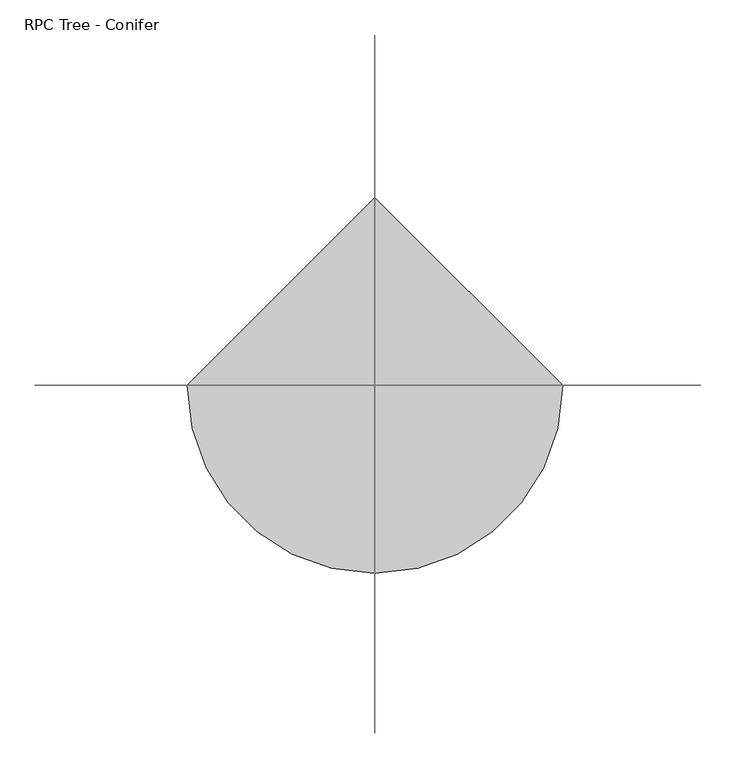
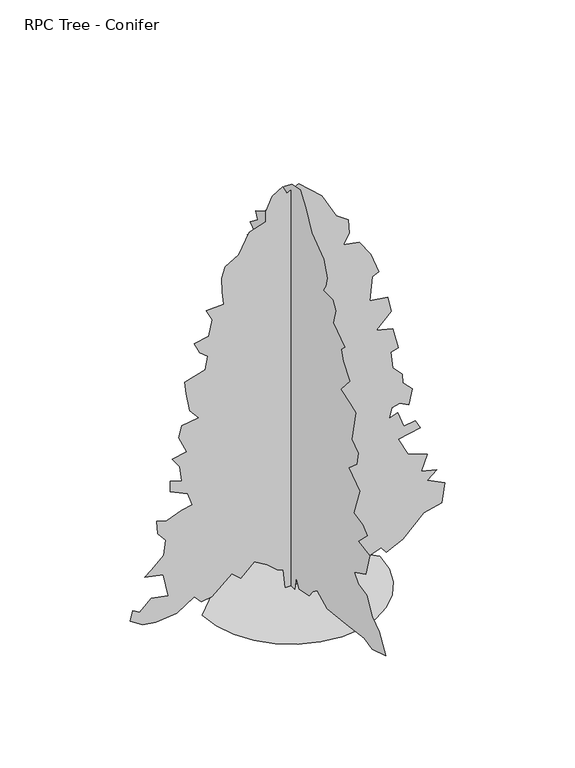
"""IFC4 building model written with IfcOpenShell, lengths in millimetres: geographic element geometry, RPC Tree - Conifer."""

from ifc_helpers import new_model, si_unit, origin, place, context, project, spatial, triangles, source, transform, mapped, element, save


def rpc_tree_conifer_9dfc94cb(model_context):
    return source(origin(), model_context, "Body", "Tessellation", [
        triangles([(0.1966724, 30.3730143, 2.21e-05), (0.196677, 46.8765628, 127.9026127), (0.1966796, 67.5060358, 185.6643395), (0.1966817, 141.7719332, 144.4061656), (0.1966847, 232.5410567, 107.2731397), (0.1966888, 335.6884489, 90.7695958), (0.1966936, 439.1223244, 95.1599346), (0.196692, 451.2137375, 24.7553998), (0.1966968, 525.4797712, 74.2660428), (0.1966987, 604.2812476, 22.1498153), (0.1967019, 661.6339605, 41.258946), (0.1967068, 773.0337742, 37.1330214), (0.1967106, 826.6693811, 86.6436667), (0.1967191, 942.1947424, 198.0422722), (0.196717, 872.0541109, 231.0490693), (0.1967148, 810.166028, 251.6794597), (0.1967121, 752.5176573, 246.8636199), (0.1967135, 740.0254692, 313.5675608), (0.196716, 756.5288223, 371.3302051), (0.1967205, 814.291503, 437.3437992), (0.1967183, 756.5288223, 449.7217501), (0.1967216, 801.9135521, 490.9809686), (0.196719, 731.7745193, 511.609833), (0.1967168, 657.5084856, 548.7436492), (0.1967174, 619.3261505, 625.1478155), (0.1967225, 715.2710936, 651.8910233), (0.1967254, 756.5288223, 689.0232771), (0.1967234, 702.8932154, 701.4011553), (0.1967209, 612.1237558, 755.038361), (0.1967249, 678.1373137, 788.0451399), (0.1967284, 683.4773947, 896.6957027), (0.1967253, 607.9967548, 907.6959034), (0.1967228, 541.9831607, 924.1993292), (0.1967255, 551.7215198, 999.3751911), (0.1967298, 632.118611, 1022.0385607), (0.1967329, 649.2560097, 1101.6127007), (0.1967296, 583.2424155, 1089.2348225), (0.1967301, 541.5533904, 1169.5343542), (0.1967339, 587.3678905, 1225.3890118), (0.1967327, 529.6052462, 1274.8992165), (0.1967366, 587.3678905, 1316.1584713), (0.1967383, 603.8712799, 1349.1651775), (0.1967356, 500.7239058, 1415.1803341), (0.1967363, 488.3459913, 1456.4379902), (0.1967412, 570.864501, 1497.697245), (0.1967412, 533.7307211, 1551.3406277), (0.1967386, 451.2137375, 1588.4652512), (0.1967428, 504.8493808, 1650.3547874), (0.1967418, 447.0867365, 1703.9843628), (0.1967401, 372.8222288, 1757.6291988), (0.1967419, 368.6952278, 1823.6488609), (0.1967455, 430.583347, 1852.5286388), (0.1967445, 385.2001433, 1885.5385426), (0.1967425, 331.562974, 1897.9133686), (0.1967471, 401.7035328, 1947.4129635), (0.1967455, 327.437499, 2005.18778), (0.1967476, 348.0663634, 2046.442384), (0.1967452, 261.422397, 2095.9572395), (0.1967443, 191.28182, 2170.2217472), (0.1967451, 145.0015871, 2265.4870079), (0.1967443, 59.2541866, 2368.2654728), (0.196743, -6.7601286, 2421.8950481), (0.1967397, -89.2778991, 2438.4), (0.196735, -147.040398, 2364.1354923), (0.1967289, -204.8027425, 2248.6162354), (0.196721, -324.4534879, 2161.9616409), (0.1967167, -357.4603031, 2067.0774616), (0.1967157, -340.9569137, 2009.3024998), (0.1967155, -320.3280493, 1972.1778763), (0.1967115, -411.0974725, 1972.1778763), (0.1967087, -439.9788128, 1922.663166), (0.1967072, -415.2229474, 1836.0238323), (0.1966997, -530.748236, 1757.6291988), (0.1967004, -493.6144561, 1724.6192951), (0.1966976, -514.2448465, 1662.7297588), (0.1966924, -580.2584407, 1584.3351254), (0.1966933, -489.4889812, 1481.1938919), (0.1966882, -585.0590198, 1451.3387375), (0.1966851, -638.021085, 1427.5582123), (0.1966813, -600.8873051, 1246.0178398), (0.1966772, -662.776914, 1200.63311), (0.1966756, -650.3990358, 1126.3670763), (0.196677, -572.0059648, 1056.2280436), (0.19667, -679.2803398, 981.9619371), (0.1966677, -617.3921843, 812.7995155), (0.1966632, -708.1616438, 796.2960897), (0.19666, -753.5463736, 759.1638359), (0.1966614, -662.776914, 668.3943764), (0.1966557, -778.3006765, 651.8910233), (0.1966535, -737.0429478, 515.7353079), (0.1966569, -625.6431341, 462.0996646), (0.1966537, -662.776914, 412.5894599), (0.1966494, -749.4193726, 396.0860704), (0.1966442, -803.0565783, 301.1896462), (0.1966395, -873.1971371, 251.6794597), (0.1966336, -935.08522, 144.4061656), (0.1966382, -803.0565783, 103.1472196), (0.1966424, -722.0818697, 121.6549744), (0.1966497, -545.8937505, 100.0198124), (0.1966574, -357.4603031, 78.3918175), (0.1966633, -258.438404, 127.9026127), (0.1966642, -217.1806752, 94.8953614), (0.1966645, -180.0468771, 49.5106453), (0.1966683, -81.0260499, 28.8813244), (0.1966712, -52.3611344, 81.269894), (0.1966695, -35.6413315, 2.01e-05), (-31.1375321, 8e-07, 2.21e-05), (-43.5151537, -1.27e-05, 111.3990688), (-76.522246, -1.22e-05, 123.7766926), (-134.2847449, -1.27e-05, 173.287951), (-208.5501882, -1.25e-05, 218.6726626), (-286.943223, 2e-06, 144.4061656), (-336.4534095, 1.4e-06, 189.7913405), (-451.9786981, 9.3e-06, 90.7695958), (-509.9897647, 1.13e-05, 83.5094103), (-550.9990711, 1.06e-05, 127.9026127), (-650.0210066, 1.65e-05, 61.888419), (-769.6717701, 2.94e-05, 49.5107997), (-843.9378038, 3.11e-05, 61.888419), (-914.0783627, 3.12e-05, 107.2731397), (-901.7004845, 2.82e-05, 165.0354751), (-860.4412296, 2.81e-05, 140.2802365), (-794.4260731, 1.45e-05, 202.1692732), (-699.5312113, 1.24e-05, 185.6643395), (-727.5164217, 7.2e-06, 321.9373624), (-831.559853, 9.3e-06, 342.4489011), (-794.4260731, 6.9e-06, 371.3302051), (-724.2870403, 1.9e-06, 437.3437992), (-711.9090895, -2.3e-06, 523.9877838), (-757.2938192, -3.4e-06, 577.6249532), (-765.5462952, -6.6e-06, 656.0164982), (-707.7836872, -7.6e-06, 639.5130724), (-621.1397026, -2.05e-05, 672.5198513), (-563.3769856, -2.28e-05, 684.8978022), (-588.132851, -2.54e-05, 759.1638359), (-687.2416271, -2.45e-05, 805.5818602), (-687.1532604, -2.74e-05, 870.5621235), (-621.1397026, -2.85e-05, 849.9332954), (-632.272526, -3.21e-05, 937.6303408), (-674.7768356, -3.35e-05, 998.4653629), (-592.258326, -3.67e-05, 1014.9687887), (-637.6430557, -3.98e-05, 1113.9891254), (-621.1397026, -4.32e-05, 1180.0042093), (-526.2447318, -5.56e-05, 1196.5076351), (-575.7549365, -5.67e-05, 1254.2702431), (-596.3838009, -6.11e-05, 1365.6685307), (-604.6362405, -6.4e-05, 1435.8091621), (-489.1109519, -6.91e-05, 1472.9414886), (-472.6075624, -7.29e-05, 1547.2105019), (-517.9922922, -7.32e-05, 1584.3351254), (-550.9990711, -7.52e-05, 1650.3547874), (-467.0983057, -8.72e-05, 1664.4822681), (-447.8516971, -9.19e-05, 1757.6291988), (-480.858476, -9.39e-05, 1823.6488609), (-381.8381029, -9.7e-05, 1827.763726), (-390.0890528, -0.0001003, 1906.1582142), (-394.2160538, -0.0001038, 1988.6828281), (-373.5856633, -0.0001072, 2050.5725098), (-297.1098262, -0.0001205, 2097.5878086), (-237.4315104, -0.0001273, 2211.4763512), (-142.5364396, -0.0001314, 2240.3561291), (-142.5364396, -0.0001342, 2302.2458107), (-105.4034228, -0.0001388, 2380.6404442), (-47.6410782, -0.0001422, 2417.7650677), (-22.8856807, -0.0001409, 2372.3803379), (43.128513, -0.0001532, 2405.3900963), (175.1564416, -0.0001518, 2285.7408588), (257.6749331, -0.0001388, 2137.2118435), (327.8155283, -0.0001475, 2087.6971333), (331.9410032, -0.0001351, 2005.18778), (298.934188, -0.0001315, 1947.4129635), (389.7036475, -0.0001335, 1930.9232723), (455.7172417, -0.0001312, 1836.0238323), (501.1019714, -0.0001272, 1716.3744495), (463.56887, -0.0001252, 1696.8520947), (447.4662918, -0.0001186, 1559.5853279), (550.6121398, -0.0001209, 1543.0805214), (571.2425303, -0.0001175, 1452.3125153), (484.5985456, -0.0001112, 1369.7956043), (579.4934801, -0.0001129, 1345.0397026), (612.5017124, -9.94e-05, 1217.1365358), (567.1155293, -9.76e-05, 1208.885586), (579.4934801, -9.36e-05, 1109.8636505), (634.0572281, -9.25e-05, 1050.2615473), (637.2560881, -9.03e-05, 998.4653629), (690.8932211, -8.95e-05, 944.8281572), (670.262867, -8.48e-05, 854.0587704), (620.7526623, -8.47e-05, 882.9400743), (575.3680052, -8.28e-05, 870.5621235), (558.8646157, -7.97e-05, 812.7995155), (608.3747841, -8.19e-05, 829.3028687), (641.381563, -7.86e-05, 734.4080069), (707.3966469, -8.12e-05, 746.785885), (736.2779509, -7.96e-05, 693.148752), (612.5017124, -7.48e-05, 668.3943764), (666.137392, -6.28e-05, 561.1200377), (777.5372057, -7.31e-05, 519.8623089), (741.8893089, -5.91e-05, 429.0943754), (831.1728853, -6.09e-05, 408.4624952), (777.5372057, -5.72e-05, 363.0777655), (876.5576151, -5.8e-05, 313.5675608), (860.0541893, -5.23e-05, 198.0422722), (756.9068516, -4.81e-05, 173.287951), (637.8229866, -3.94e-05, 57.4519029), (542.3611899, -2.57e-05, 12.3776227), (513.479886, -2.65e-05, 49.5106453), (405.178357, -2.16e-05, 12.7724149), (290.6817302, -1.8e-05, 8.2517589), (245.2970186, -1.85e-05, 49.5106453), (142.1498081, -1.71e-05, 86.6436667), (44.8004949, -1.33e-05, 66.7016699), (34.8766616, -1e-05, 2.01e-05), (-504.8127188, -2.8e-06, 3.62e-05), (-491.4609538, -115.7145757, 3.24e-05), (-453.4386744, -221.9797464, 2.81e-05), (-393.7878096, -315.7514754, 2.35e-05), (-315.5547941, -393.9844909, 1.88e-05), (-221.7830832, -453.6353557, 1.42e-05), (-115.5179035, -491.6576351, 9.9e-06), (0.1966932, -505.0094001, 6.1e-06), (115.9112479, -491.6576351, 3.1e-06), (222.1764095, -453.6353557, 1e-06), (315.9481567, -393.9844909, 0.0), (394.1811722, -315.7514754, 0.0), (453.832037, -221.9797464, 1e-06), (491.8543164, -115.7145757, 3.1e-06), (505.2060814, 4.68e-05, 6.1e-06), (0.1966049, 505.0094001, 3.62e-05)], [[26, 27, 28], [21, 22, 23], [19, 20, 21], [51, 52, 53], [7, 8, 9], [35, 36, 37], [13, 14, 15], [34, 35, 37], [54, 55, 56], [72, 73, 74], [95, 96, 97], [88, 89, 90], [44, 45, 46], [86, 87, 88], [85, 86, 88], [51, 53, 54], [44, 46, 47], [88, 90, 91], [13, 15, 16], [13, 16, 17], [38, 39, 40], [25, 26, 28], [25, 28, 29], [47, 48, 49], [56, 57, 58], [30, 31, 32], [29, 30, 32], [41, 42, 43], [40, 41, 43], [106, 1, 2], [105, 106, 2], [75, 76, 77], [94, 95, 97], [94, 97, 98], [78, 79, 80], [83, 84, 85], [29, 32, 33], [103, 104, 105], [12, 13, 17], [11, 12, 17], [77, 78, 80], [102, 103, 105], [62, 63, 64], [80, 81, 82], [80, 82, 83], [61, 62, 64], [61, 64, 65], [60, 61, 65], [59, 60, 65], [69, 70, 71], [69, 71, 72], [94, 98, 99], [93, 94, 99], [92, 93, 99], [92, 99, 100], [91, 92, 100], [91, 100, 101], [47, 49, 50], [9, 10, 11], [9, 11, 17], [9, 17, 18], [7, 9, 18], [59, 65, 66], [59, 66, 67], [59, 67, 68], [59, 68, 69], [58, 59, 69], [56, 58, 69], [54, 56, 69], [54, 69, 72], [51, 54, 72], [50, 51, 72], [50, 72, 74], [50, 74, 75], [50, 75, 77], [47, 50, 77], [44, 47, 77], [43, 44, 77], [40, 43, 77], [40, 77, 80], [40, 80, 83], [38, 40, 83], [38, 83, 85], [37, 38, 85], [34, 37, 85], [33, 34, 85], [29, 33, 85], [25, 29, 85], [25, 85, 88], [25, 88, 91], [25, 91, 101], [25, 101, 102], [24, 25, 102], [23, 24, 102], [21, 23, 102], [105, 2, 3], [102, 105, 3], [21, 102, 3], [21, 3, 4], [21, 4, 5], [21, 5, 6], [21, 6, 7], [21, 7, 18], [19, 21, 18], [125, 126, 127], [198, 199, 200], [153, 154, 155], [139, 140, 141], [130, 131, 132], [120, 121, 122], [119, 120, 122], [186, 187, 188], [136, 137, 138], [135, 136, 138], [150, 151, 152], [193, 194, 195], [192, 193, 195], [125, 127, 128], [180, 181, 182], [163, 164, 165], [185, 186, 188], [196, 197, 198], [190, 191, 192], [111, 112, 113], [212, 107, 108], [211, 212, 108], [173, 174, 175], [149, 150, 152], [179, 180, 182], [129, 130, 132], [146, 147, 148], [204, 205, 206], [200, 201, 202], [200, 202, 203], [162, 163, 165], [190, 192, 195], [165, 166, 167], [118, 119, 122], [118, 122, 123], [118, 123, 124], [117, 118, 124], [116, 117, 124], [176, 177, 178], [176, 178, 179], [129, 132, 133], [185, 188, 189], [142, 143, 144], [141, 142, 144], [161, 162, 165], [161, 165, 167], [161, 167, 168], [116, 124, 125], [145, 146, 148], [144, 145, 148], [114, 115, 116], [113, 114, 116], [113, 116, 125], [113, 125, 128], [113, 128, 129], [113, 129, 133], [113, 133, 134], [111, 113, 134], [168, 169, 170], [168, 170, 171], [161, 168, 171], [160, 161, 171], [159, 160, 171], [158, 159, 171], [157, 158, 171], [156, 157, 171], [155, 156, 171], [171, 172, 173], [171, 173, 175], [155, 171, 175], [155, 175, 176], [153, 155, 176], [152, 153, 176], [149, 152, 176], [149, 176, 179], [148, 149, 179], [144, 148, 179], [144, 179, 182], [144, 182, 183], [141, 144, 183], [139, 141, 183], [138, 139, 183], [135, 138, 183], [134, 135, 183], [111, 134, 183], [110, 111, 183], [110, 183, 184], [110, 184, 185], [110, 185, 189], [110, 189, 190], [110, 190, 195], [109, 110, 195], [108, 109, 195], [211, 108, 195], [210, 211, 195], [210, 195, 196], [209, 210, 196], [209, 196, 198], [208, 209, 198], [207, 208, 198], [206, 207, 198], [204, 206, 198], [203, 204, 198], [200, 203, 198], [227, 228, 213], [226, 227, 213], [226, 213, 214], [225, 226, 214], [225, 214, 215], [225, 215, 216], [224, 225, 216], [223, 224, 216], [223, 216, 217], [223, 217, 218], [223, 218, 219], [223, 219, 220], [223, 220, 221], [223, 221, 222]], closed=False),
    ])


if __name__ == "__main__":
    model = new_model("IFC4")
    model_context = context("Model", 3, world=origin())
    ifc_project = project(units=[si_unit("LENGTHUNIT", "METRE", prefix="MILLI")], contexts=[model_context])
    site = spatial("IfcSite", under=ifc_project)
    building = spatial("IfcBuilding", under=site)
    placement = place(None, origin())
    rpc_tree_conifer_shape = rpc_tree_conifer_9dfc94cb(model_context)
    element("IfcGeographicElement", 1, ObjectType="RPC Tree - Conifer", at=placement, inside=building, context=model_context, shape_type="MappedRepresentation", body=[
        mapped(rpc_tree_conifer_shape, transform((0.0, 0.0, 0.0), x_axis=(1.0, 0.0, 0.0), y_axis=(0.0, 1.0, 0.0), z_axis=(0.0, 0.0, 1.0))),
    ])
    save(model, "model.ifc")

# Revit data of these elements
# Type "RPC Tree - Conifer"
#   built-in parameter 1005198 = "{2, 15},{39, RPC-16-G0M4-N9PX-U6TN-C000-ST1L-LVER-AU},{1, 0},{1, 0},{2, 13},{1, 8},{5, Color},{1, 0},{1, 0},{3, 0.8},{3, 0.8},{3, 0.8},{1, 8},{7, BBoxMin},{1, 0},{1, 0},{1, 0},{1, 0},{1, 0},{1, 8},{7, BBoxMax},{1, 0},{1, 0},{1, 0},{1, 0},{1, 0},{2, 11},{9, RPCTypeId},{1, 0},{1, 0},{39, RPC-16-G0M4-N9PX-U6TN-C000-ST1L-LVER-AU},{1, 6},{14, RPCPlantHeight},{1, 0},{1, 0},{2, 13},{2, 11},{7, keyword},{1, 0},{1, 0},{34, :RPCs:Trees [General]:Geometry:RPC},{2, 11},{8, category},{1, 0},{1, 0},{15, Trees [General]},{2, 11},{12, LocalizedUID},{1, 0},{1, 0},{15, Colorado Spruce},{2, 14},{6, Height},{1, 0},{1, 0},{2, 13},{1, 2},{16, Cast Reflections},{1, 0},{1, 0},{1, 0},{1, 2},{12, Cast Shadows},{1, 0},{1, 0},{1, 1},{1, 2},{9, Lock View},{1, 0},{1, 0},{1, 0},{1, 4},{5, ViewC},{1, 0},{1, 0},{1, 0},{21, assetlibrary_base.fbx},{1, 5},"
#   built-in parameter 1005195 = "RPC-16-G0M4-N9PX-U6TN-C000-ST1L-LVER-AU"
#   Assembly Code = "G2050500"
#   Height = 8' - 0"
#   Description = (empty or 0)
#   Default Elevation = 0
